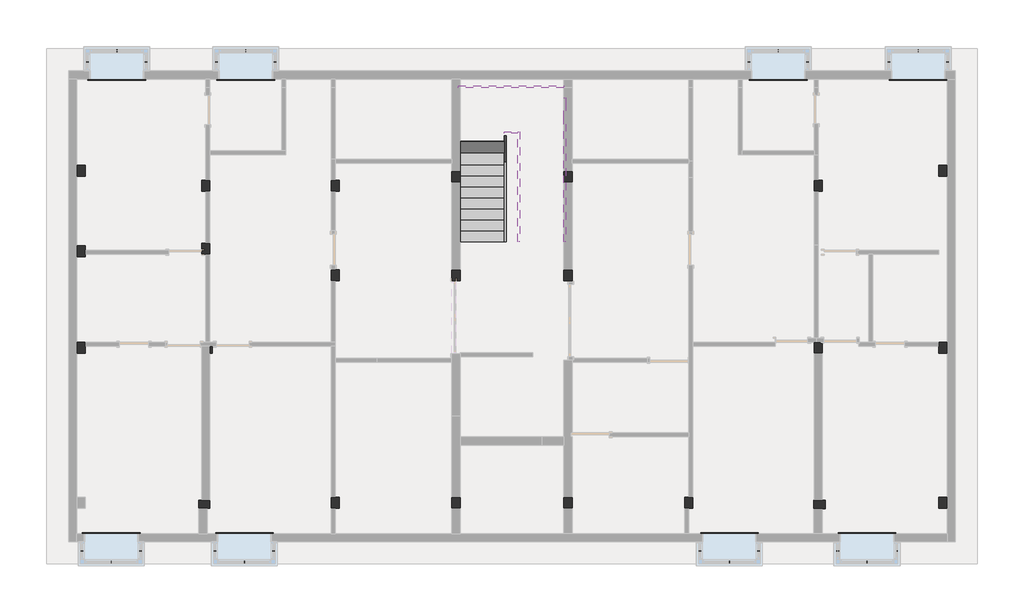
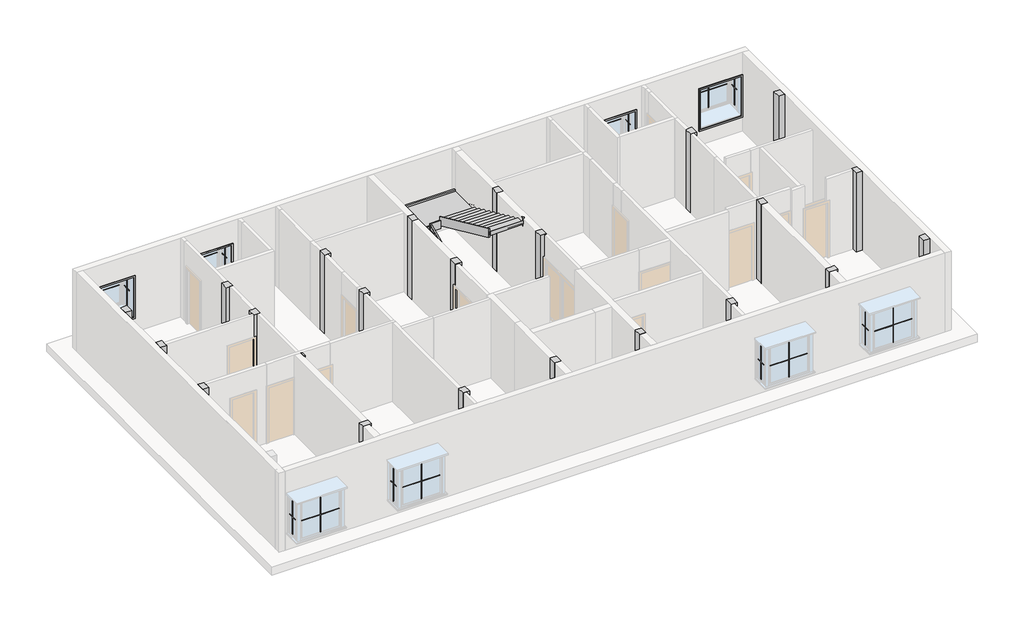
# One storey, part 3 of 3: 32 proxies, 23 columns, 6 members, 1 stair flight.
"""IFC4 building model written with IfcOpenShell, lengths in millimetres."""

from ifc_helpers import new_model, si_unit, frame, origin, place, context, project, spatial, polyline, outline, extrude, faceted_brep, transform, mapped, element, save
from components import m_muntin_pattern_2x2_m_muntin_pattern_2x2_c1fd4460, m_muntin_pattern_2x2_m_muntin_pattern_2x2_777b163a, m_trim_window_interior_flat_picture_frame_44e8afef, stair_flight_7d9339af

model = new_model("IFC4")

# Units and contexts
model_context = context("Model", 3, world=origin())
ifc_project = project(units=[si_unit("LENGTHUNIT", "METRE", prefix="MILLI")], contexts=[model_context])

# Site, building, storey
site = spatial("IfcSite", under=ifc_project)
building = spatial("IfcBuilding", under=site)
storey = spatial("IfcBuildingStorey", under=building, Elevation=19202.4)

# Proxies
placement = place(None, origin())
m_muntin_pattern_2x2_m_muntin_pattern_2x2_shape = m_muntin_pattern_2x2_m_muntin_pattern_2x2_c1fd4460(model_context)
element("IfcBuildingElementProxy", 1, Name="M_Muntin Pattern_2x2 : M_Muntin Pattern_2x2", ObjectType="M_Muntin Pattern_2x2 : M_Muntin Pattern_2x2", at=placement, inside=storey, context=model_context, shape_type="MappedRepresentation", body=[
    mapped(m_muntin_pattern_2x2_m_muntin_pattern_2x2_shape, transform((-11500.7987957, -5499.9182661, 19923.05), x_axis=(-1.0, 0.0, 0.0), y_axis=(0.0, -1.0, 0.0), z_axis=(0.0, 0.0, 1.0))),
])
element("IfcBuildingElementProxy", 2, Name="M_Muntin Pattern_2x2 : M_Muntin Pattern_2x2", ObjectType="M_Muntin Pattern_2x2 : M_Muntin Pattern_2x2", at=placement, inside=storey, context=model_context, shape_type="MappedRepresentation", body=[
    mapped(m_muntin_pattern_2x2_m_muntin_pattern_2x2_shape, transform((-7819.250543, -5499.9182661, 19923.05), x_axis=(-1.0, 0.0, 0.0), y_axis=(0.0, -1.0, 0.0), z_axis=(0.0, 0.0, 1.0))),
])
element("IfcBuildingElementProxy", 3, Name="M_Muntin Pattern_2x2 : M_Muntin Pattern_2x2", ObjectType="M_Muntin Pattern_2x2 : M_Muntin Pattern_2x2", at=placement, inside=storey, context=model_context, shape_type="MappedRepresentation", body=[
    mapped(m_muntin_pattern_2x2_m_muntin_pattern_2x2_shape, transform((5599.7512082, -5499.9182661, 19923.05), x_axis=(-1.0, 0.0, 0.0), y_axis=(0.0, -1.0, 0.0), z_axis=(0.0, 0.0, 1.0))),
])
element("IfcBuildingElementProxy", 4, Name="M_Muntin Pattern_2x2 : M_Muntin Pattern_2x2", ObjectType="M_Muntin Pattern_2x2 : M_Muntin Pattern_2x2", at=placement, inside=storey, context=model_context, shape_type="MappedRepresentation", body=[
    mapped(m_muntin_pattern_2x2_m_muntin_pattern_2x2_shape, transform((9408.6146942, -5499.9182662, 19923.05), x_axis=(-1.0, 0.0, 0.0), y_axis=(0.0, -1.0, 0.0), z_axis=(0.0, 0.0, 1.0))),
])
element("IfcBuildingElementProxy", 5, Name="M_Muntin Pattern_2x2 : M_Muntin Pattern_2x2", ObjectType="M_Muntin Pattern_2x2 : M_Muntin Pattern_2x2", at=placement, inside=storey, context=model_context, shape_type="MappedRepresentation", body=[
    mapped(m_muntin_pattern_2x2_m_muntin_pattern_2x2_shape, transform((-11348.3987957, 8647.7317329, 19923.05), x_axis=(1.0, 0.0, 0.0), y_axis=(0.0, 1.0, 0.0), z_axis=(0.0, 0.0, 1.0))),
])
element("IfcBuildingElementProxy", 6, Name="M_Muntin Pattern_2x2 : M_Muntin Pattern_2x2", ObjectType="M_Muntin Pattern_2x2 : M_Muntin Pattern_2x2", at=placement, inside=storey, context=model_context, shape_type="MappedRepresentation", body=[
    mapped(m_muntin_pattern_2x2_m_muntin_pattern_2x2_shape, transform((-7779.6987993, 8647.7317329, 19923.05), x_axis=(1.0, 0.0, 0.0), y_axis=(0.0, 1.0, 0.0), z_axis=(0.0, 0.0, 1.0))),
])
element("IfcBuildingElementProxy", 7, Name="M_Muntin Pattern_2x2 : M_Muntin Pattern_2x2", ObjectType="M_Muntin Pattern_2x2 : M_Muntin Pattern_2x2", at=placement, inside=storey, context=model_context, shape_type="MappedRepresentation", body=[
    mapped(m_muntin_pattern_2x2_m_muntin_pattern_2x2_shape, transform((6952.301208, 8647.7317329, 19923.05), x_axis=(1.0, 0.0, 0.0), y_axis=(0.0, 1.0, 0.0), z_axis=(0.0, 0.0, 1.0))),
])
element("IfcBuildingElementProxy", 8, Name="M_Muntin Pattern_2x2 : M_Muntin Pattern_2x2", ObjectType="M_Muntin Pattern_2x2 : M_Muntin Pattern_2x2", at=placement, inside=storey, context=model_context, shape_type="MappedRepresentation", body=[
    mapped(m_muntin_pattern_2x2_m_muntin_pattern_2x2_shape, transform((10825.8012075, 8647.7317329, 19923.05), x_axis=(1.0, 0.0, 0.0), y_axis=(0.0, 1.0, 0.0), z_axis=(0.0, 0.0, 1.0))),
])
m_muntin_pattern_2x2_m_muntin_pattern_2x2_2_shape = m_muntin_pattern_2x2_m_muntin_pattern_2x2_777b163a(model_context)
element("IfcBuildingElementProxy", 9, Name="M_Muntin Pattern_2x2 : M_Muntin Pattern_2x2", ObjectType="M_Muntin Pattern_2x2 : M_Muntin Pattern_2x2", at=placement, inside=storey, context=model_context, shape_type="MappedRepresentation", body=[
    mapped(m_muntin_pattern_2x2_m_muntin_pattern_2x2_2_shape, transform((-10690.4737957, -5190.3932661, 19923.05), x_axis=(0.0, 1.0, 0.0), y_axis=(-1.0, 0.0, 0.0), z_axis=(0.0, 0.0, 1.0))),
])
element("IfcBuildingElementProxy", 10, Name="M_Muntin Pattern_2x2 : M_Muntin Pattern_2x2", ObjectType="M_Muntin Pattern_2x2 : M_Muntin Pattern_2x2", at=placement, inside=storey, context=model_context, shape_type="MappedRepresentation", body=[
    mapped(m_muntin_pattern_2x2_m_muntin_pattern_2x2_2_shape, transform((-12311.1237957, -5190.3932661, 19923.05), x_axis=(0.0, -1.0, 0.0), y_axis=(1.0, 0.0, 0.0), z_axis=(0.0, 0.0, 1.0))),
])
element("IfcBuildingElementProxy", 11, Name="M_Muntin Pattern_2x2 : M_Muntin Pattern_2x2", ObjectType="M_Muntin Pattern_2x2 : M_Muntin Pattern_2x2", at=placement, inside=storey, context=model_context, shape_type="MappedRepresentation", body=[
    mapped(m_muntin_pattern_2x2_m_muntin_pattern_2x2_2_shape, transform((-7008.925543, -5190.3932661, 19923.05), x_axis=(0.0, 1.0, 0.0), y_axis=(-1.0, 0.0, 0.0), z_axis=(0.0, 0.0, 1.0))),
])
element("IfcBuildingElementProxy", 12, Name="M_Muntin Pattern_2x2 : M_Muntin Pattern_2x2", ObjectType="M_Muntin Pattern_2x2 : M_Muntin Pattern_2x2", at=placement, inside=storey, context=model_context, shape_type="MappedRepresentation", body=[
    mapped(m_muntin_pattern_2x2_m_muntin_pattern_2x2_2_shape, transform((-8629.575543, -5190.3932661, 19923.05), x_axis=(0.0, -1.0, 0.0), y_axis=(1.0, 0.0, 0.0), z_axis=(0.0, 0.0, 1.0))),
])
element("IfcBuildingElementProxy", 13, Name="M_Muntin Pattern_2x2 : M_Muntin Pattern_2x2", ObjectType="M_Muntin Pattern_2x2 : M_Muntin Pattern_2x2", at=placement, inside=storey, context=model_context, shape_type="MappedRepresentation", body=[
    mapped(m_muntin_pattern_2x2_m_muntin_pattern_2x2_2_shape, transform((6410.0762082, -5190.3932661, 19923.05), x_axis=(0.0, 1.0, 0.0), y_axis=(-1.0, 0.0, 0.0), z_axis=(0.0, 0.0, 1.0))),
])
element("IfcBuildingElementProxy", 14, Name="M_Muntin Pattern_2x2 : M_Muntin Pattern_2x2", ObjectType="M_Muntin Pattern_2x2 : M_Muntin Pattern_2x2", at=placement, inside=storey, context=model_context, shape_type="MappedRepresentation", body=[
    mapped(m_muntin_pattern_2x2_m_muntin_pattern_2x2_2_shape, transform((4789.4262082, -5190.3932661, 19923.05), x_axis=(0.0, -1.0, 0.0), y_axis=(1.0, 0.0, 0.0), z_axis=(0.0, 0.0, 1.0))),
])
element("IfcBuildingElementProxy", 15, Name="M_Muntin Pattern_2x2 : M_Muntin Pattern_2x2", ObjectType="M_Muntin Pattern_2x2 : M_Muntin Pattern_2x2", at=placement, inside=storey, context=model_context, shape_type="MappedRepresentation", body=[
    mapped(m_muntin_pattern_2x2_m_muntin_pattern_2x2_2_shape, transform((10218.9396942, -5190.3932662, 19923.05), x_axis=(0.0, 1.0, 0.0), y_axis=(-1.0, 0.0, 0.0), z_axis=(0.0, 0.0, 1.0))),
])
element("IfcBuildingElementProxy", 16, Name="M_Muntin Pattern_2x2 : M_Muntin Pattern_2x2", ObjectType="M_Muntin Pattern_2x2 : M_Muntin Pattern_2x2", at=placement, inside=storey, context=model_context, shape_type="MappedRepresentation", body=[
    mapped(m_muntin_pattern_2x2_m_muntin_pattern_2x2_2_shape, transform((8598.2896942, -5190.3932661, 19923.05), x_axis=(0.0, -1.0, 0.0), y_axis=(1.0, 0.0, 0.0), z_axis=(0.0, 0.0, 1.0))),
])
element("IfcBuildingElementProxy", 17, Name="M_Muntin Pattern_2x2 : M_Muntin Pattern_2x2", ObjectType="M_Muntin Pattern_2x2 : M_Muntin Pattern_2x2", at=placement, inside=storey, context=model_context, shape_type="MappedRepresentation", body=[
    mapped(m_muntin_pattern_2x2_m_muntin_pattern_2x2_2_shape, transform((-12158.7237957, 8338.2067329, 19923.05), x_axis=(0.0, -1.0, 0.0), y_axis=(1.0, 0.0, 0.0), z_axis=(0.0, 0.0, 1.0))),
])
element("IfcBuildingElementProxy", 18, Name="M_Muntin Pattern_2x2 : M_Muntin Pattern_2x2", ObjectType="M_Muntin Pattern_2x2 : M_Muntin Pattern_2x2", at=placement, inside=storey, context=model_context, shape_type="MappedRepresentation", body=[
    mapped(m_muntin_pattern_2x2_m_muntin_pattern_2x2_2_shape, transform((-10538.0737957, 8338.2067329, 19923.05), x_axis=(0.0, 1.0, 0.0), y_axis=(-1.0, 0.0, 0.0), z_axis=(0.0, 0.0, 1.0))),
])
element("IfcBuildingElementProxy", 19, Name="M_Muntin Pattern_2x2 : M_Muntin Pattern_2x2", ObjectType="M_Muntin Pattern_2x2 : M_Muntin Pattern_2x2", at=placement, inside=storey, context=model_context, shape_type="MappedRepresentation", body=[
    mapped(m_muntin_pattern_2x2_m_muntin_pattern_2x2_2_shape, transform((-8590.0237993, 8338.2067329, 19923.05), x_axis=(0.0, -1.0, 0.0), y_axis=(1.0, 0.0, 0.0), z_axis=(0.0, 0.0, 1.0))),
])
element("IfcBuildingElementProxy", 20, Name="M_Muntin Pattern_2x2 : M_Muntin Pattern_2x2", ObjectType="M_Muntin Pattern_2x2 : M_Muntin Pattern_2x2", at=placement, inside=storey, context=model_context, shape_type="MappedRepresentation", body=[
    mapped(m_muntin_pattern_2x2_m_muntin_pattern_2x2_2_shape, transform((-6969.3737993, 8338.2067329, 19923.05), x_axis=(0.0, 1.0, 0.0), y_axis=(-1.0, 0.0, 0.0), z_axis=(0.0, 0.0, 1.0))),
])
element("IfcBuildingElementProxy", 21, Name="M_Muntin Pattern_2x2 : M_Muntin Pattern_2x2", ObjectType="M_Muntin Pattern_2x2 : M_Muntin Pattern_2x2", at=placement, inside=storey, context=model_context, shape_type="MappedRepresentation", body=[
    mapped(m_muntin_pattern_2x2_m_muntin_pattern_2x2_2_shape, transform((6141.976208, 8338.2067329, 19923.05), x_axis=(0.0, -1.0, 0.0), y_axis=(1.0, 0.0, 0.0), z_axis=(0.0, 0.0, 1.0))),
])
element("IfcBuildingElementProxy", 22, Name="M_Muntin Pattern_2x2 : M_Muntin Pattern_2x2", ObjectType="M_Muntin Pattern_2x2 : M_Muntin Pattern_2x2", at=placement, inside=storey, context=model_context, shape_type="MappedRepresentation", body=[
    mapped(m_muntin_pattern_2x2_m_muntin_pattern_2x2_2_shape, transform((7762.626208, 8338.2067329, 19923.05), x_axis=(0.0, 1.0, 0.0), y_axis=(-1.0, 0.0, 0.0), z_axis=(0.0, 0.0, 1.0))),
])
element("IfcBuildingElementProxy", 23, Name="M_Muntin Pattern_2x2 : M_Muntin Pattern_2x2", ObjectType="M_Muntin Pattern_2x2 : M_Muntin Pattern_2x2", at=placement, inside=storey, context=model_context, shape_type="MappedRepresentation", body=[
    mapped(m_muntin_pattern_2x2_m_muntin_pattern_2x2_2_shape, transform((10015.4762075, 8338.2067329, 19923.05), x_axis=(0.0, -1.0, 0.0), y_axis=(1.0, 0.0, 0.0), z_axis=(0.0, 0.0, 1.0))),
])
element("IfcBuildingElementProxy", 24, Name="M_Muntin Pattern_2x2 : M_Muntin Pattern_2x2", ObjectType="M_Muntin Pattern_2x2 : M_Muntin Pattern_2x2", at=placement, inside=storey, context=model_context, shape_type="MappedRepresentation", body=[
    mapped(m_muntin_pattern_2x2_m_muntin_pattern_2x2_2_shape, transform((11636.1262075, 8338.2067329, 19923.05), x_axis=(0.0, 1.0, 0.0), y_axis=(-1.0, 0.0, 0.0), z_axis=(0.0, 0.0, 1.0))),
])
m_trim_window_interior_flat_picture_frame_shape = m_trim_window_interior_flat_picture_frame_44e8afef(model_context)
element("IfcBuildingElementProxy", 25, Name="M_Trim-Window-Interior-Flat : Picture Frame", ObjectType="M_Trim-Window-Interior-Flat : Picture Frame", at=placement, inside=storey, context=model_context, shape_type="MappedRepresentation", body=[
    mapped(m_trim_window_interior_flat_picture_frame_shape, transform((-11500.7987957, -4712.5932661, 21353.2), x_axis=(-1.0, 0.0, 0.0), y_axis=(0.0, 0.0, 1.0), z_axis=(0.0, 1.0, 0.0))),
])
element("IfcBuildingElementProxy", 26, Name="M_Trim-Window-Interior-Flat : Picture Frame", ObjectType="M_Trim-Window-Interior-Flat : Picture Frame", at=placement, inside=storey, context=model_context, shape_type="MappedRepresentation", body=[
    mapped(m_trim_window_interior_flat_picture_frame_shape, transform((-7819.250543, -4712.5932661, 21353.2), x_axis=(-1.0, 0.0, 0.0), y_axis=(0.0, 0.0, 1.0), z_axis=(0.0, 1.0, 0.0))),
])
element("IfcBuildingElementProxy", 27, Name="M_Trim-Window-Interior-Flat : Picture Frame", ObjectType="M_Trim-Window-Interior-Flat : Picture Frame", at=placement, inside=storey, context=model_context, shape_type="MappedRepresentation", body=[
    mapped(m_trim_window_interior_flat_picture_frame_shape, transform((5599.7512082, -4712.5932661, 21353.2), x_axis=(-1.0, 0.0, 0.0), y_axis=(0.0, 0.0, 1.0), z_axis=(0.0, 1.0, 0.0))),
])
element("IfcBuildingElementProxy", 28, Name="M_Trim-Window-Interior-Flat : Picture Frame", ObjectType="M_Trim-Window-Interior-Flat : Picture Frame", at=placement, inside=storey, context=model_context, shape_type="MappedRepresentation", body=[
    mapped(m_trim_window_interior_flat_picture_frame_shape, transform((9408.6146942, -4712.5932661, 21353.2), x_axis=(-1.0, 0.0, 0.0), y_axis=(0.0, 0.0, 1.0), z_axis=(0.0, 1.0, 0.0))),
])
element("IfcBuildingElementProxy", 29, Name="M_Trim-Window-Interior-Flat : Picture Frame", ObjectType="M_Trim-Window-Interior-Flat : Picture Frame", at=placement, inside=storey, context=model_context, shape_type="MappedRepresentation", body=[
    mapped(m_trim_window_interior_flat_picture_frame_shape, transform((-11348.3987957, 7860.4067329, 21353.2), x_axis=(1.0, 0.0, 0.0), y_axis=(0.0, 0.0, 1.0), z_axis=(0.0, -1.0, 0.0))),
])
element("IfcBuildingElementProxy", 30, Name="M_Trim-Window-Interior-Flat : Picture Frame", ObjectType="M_Trim-Window-Interior-Flat : Picture Frame", at=placement, inside=storey, context=model_context, shape_type="MappedRepresentation", body=[
    mapped(m_trim_window_interior_flat_picture_frame_shape, transform((-7779.6987993, 7860.4067329, 21353.2), x_axis=(1.0, 0.0, 0.0), y_axis=(0.0, 0.0, 1.0), z_axis=(0.0, -1.0, 0.0))),
])
element("IfcBuildingElementProxy", 31, Name="M_Trim-Window-Interior-Flat : Picture Frame", ObjectType="M_Trim-Window-Interior-Flat : Picture Frame", at=placement, inside=storey, context=model_context, shape_type="MappedRepresentation", body=[
    mapped(m_trim_window_interior_flat_picture_frame_shape, transform((6952.301208, 7860.4067329, 21353.2), x_axis=(1.0, 0.0, 0.0), y_axis=(0.0, 0.0, 1.0), z_axis=(0.0, -1.0, 0.0))),
])
element("IfcBuildingElementProxy", 32, Name="M_Trim-Window-Interior-Flat : Picture Frame", ObjectType="M_Trim-Window-Interior-Flat : Picture Frame", at=placement, inside=storey, context=model_context, shape_type="MappedRepresentation", body=[
    mapped(m_trim_window_interior_flat_picture_frame_shape, transform((10825.8012075, 7860.4067329, 21353.2), x_axis=(1.0, 0.0, 0.0), y_axis=(0.0, 0.0, 1.0), z_axis=(0.0, -1.0, 0.0))),
])

# Columns
element("IfcColumn", 33, ObjectType="Rectangular Column : 1'X 9\"", at=placement, inside=storey, context=model_context, shape_type="SweptSolid", body=[
    extrude(outline(polyline([(-12224.6987957, 583.3067334), (-12224.6987957, 278.5067334), (-12453.2987957, 278.5067334), (-12453.2987957, 583.3067334), (-12224.6987957, 583.3067334)])), frame((0.0, 0.0, 19202.4), z_axis=(0.0, 0.0, 1.0), x_axis=(1.0, 0.0, 0.0)), (0.0, 0.0, 1.0), 3048.0),
])
element("IfcColumn", 34, ObjectType="Rectangular Column : 1'X 9\"", at=placement, inside=storey, context=model_context, shape_type="SweptSolid", body=[
    extrude(outline(polyline([(-12224.6987957, 3256.6567332), (-12224.6987957, 2951.8567332), (-12453.2987957, 2951.8567332), (-12453.2987957, 3256.6567332), (-12224.6987957, 3256.6567332)])), frame((0.0, 0.0, 19202.4), z_axis=(0.0, 0.0, 1.0), x_axis=(1.0, 0.0, 0.0)), (0.0, 0.0, 1.0), 3048.0),
])
element("IfcColumn", 35, ObjectType="Rectangular Column : 1'X 9\"", at=placement, inside=storey, context=model_context, shape_type="Brep", body=[
    faceted_brep([(-8770.2987992, 5066.406733, 19202.4), (-8770.2987992, 4761.606733, 19202.4), (-8884.5987992, 4761.606733, 19202.4), (-8998.8987992, 4761.606733, 19202.4), (-8998.8987992, 5066.406733, 19202.4), (-8884.5987992, 5066.406733, 19202.4), (-8770.2987992, 5066.406733, 22250.4), (-8770.2987992, 4761.606733, 22250.4), (-8884.5987992, 4761.606733, 22250.4), (-8998.8987992, 4761.606733, 22250.4), (-8998.8987992, 5066.406733, 22250.4), (-8884.5987992, 5066.406733, 22250.4)], [[[0, 1, 2, 3, 4, 5]], [[6, 7, 1, 0]], [[7, 8, 9, 3, 2, 1]], [[9, 10, 4, 3]], [[10, 11, 6, 0, 5, 4]], [[6, 11, 10, 9, 8, 7]]]),
])
element("IfcColumn", 36, ObjectType="Rectangular Column : 1'X 9\"", at=placement, inside=storey, context=model_context, shape_type="Brep", body=[
    faceted_brep([(-8770.2987992, 3326.5067332, 19202.4), (-8770.2987992, 3021.7067332, 19202.4), (-8884.598796, 3021.7067332, 19202.4), (-8998.8987992, 3021.7067332, 19202.4), (-8998.8987992, 3326.5067332, 19202.4), (-8884.5987992, 3326.5067332, 19202.4), (-8770.2987992, 3326.5067332, 22250.4), (-8770.2987992, 3021.7067332, 22250.4), (-8884.598796, 3021.7067332, 22250.4), (-8998.8987992, 3021.7067332, 22250.4), (-8998.8987992, 3326.5067332, 22250.4), (-8884.5987992, 3326.5067332, 22250.4)], [[[0, 1, 2, 3, 4, 5]], [[6, 7, 1, 0]], [[7, 8, 9, 3, 2, 1]], [[9, 10, 4, 3]], [[10, 11, 6, 0, 5, 4]], [[6, 11, 10, 9, 8, 7]]]),
])
element("IfcColumn", 37, ObjectType="Rectangular Column : 1'X 9\"", at=placement, inside=storey, context=model_context, shape_type="SweptSolid", body=[
    extrude(outline(polyline([(-8713.148796, 278.5067334), (-8771.750543, 278.5067334), (-8771.750543, 469.0067334), (-8713.148796, 469.0067334), (-8713.148796, 278.5067334)])), frame((0.0, 0.0, 19202.4), z_axis=(0.0, 0.0, 1.0), x_axis=(1.0, 0.0, 0.0)), (0.0, 0.0, 1.0), 3048.0),
])
element("IfcColumn", 38, ObjectType="Rectangular Column : 1'X 9\"", at=placement, inside=storey, context=model_context, shape_type="Brep", body=[
    faceted_brep([(-5188.8987995, 5066.406733, 19202.4), (-5188.8987995, 4761.606733, 19202.4), (-5303.1987995, 4761.606733, 19202.4), (-5417.4987995, 4761.606733, 19202.4), (-5417.4987995, 5066.406733, 19202.4), (-5303.1987995, 5066.406733, 19202.4), (-5188.8987995, 5066.406733, 22250.4), (-5188.8987995, 4761.606733, 22250.4), (-5303.1987995, 4761.606733, 22250.4), (-5417.4987995, 4761.606733, 22250.4), (-5417.4987995, 5066.406733, 22250.4), (-5303.1987995, 5066.406733, 22250.4)], [[[0, 1, 2, 3, 4, 5]], [[6, 7, 1, 0]], [[7, 8, 9, 3, 2, 1]], [[9, 10, 4, 3]], [[10, 11, 6, 0, 5, 4]], [[6, 11, 10, 9, 8, 7]]]),
])
element("IfcColumn", 39, ObjectType="Rectangular Column : 1'X 9\"", at=placement, inside=storey, context=model_context, shape_type="Brep", body=[
    faceted_brep([(-5188.8987995, 2589.9067802, 19202.4), (-5188.8987995, 2285.1067802, 19202.4), (-5303.1987995, 2285.1067802, 19202.4), (-5417.4987995, 2285.1067802, 19202.4), (-5417.4987995, 2589.9067802, 19202.4), (-5303.1987995, 2589.9067802, 19202.4), (-5188.8987995, 2589.9067802, 22250.4), (-5188.8987995, 2285.1067802, 22250.4), (-5303.1987995, 2285.1067802, 22250.4), (-5417.4987995, 2285.1067802, 22250.4), (-5417.4987995, 2589.9067802, 22250.4), (-5303.1987995, 2589.9067802, 22250.4)], [[[0, 1, 2, 3, 4, 5]], [[6, 7, 1, 0]], [[7, 8, 9, 3, 2, 1]], [[9, 10, 4, 3]], [[10, 11, 6, 0, 5, 4]], [[6, 11, 10, 9, 8, 7]]]),
])
element("IfcColumn", 40, ObjectType="Rectangular Column : 1'X 9\"", at=placement, inside=storey, context=model_context, shape_type="Brep", body=[
    faceted_brep([(-5188.8987963, -3709.2932193, 19202.4), (-5188.8987963, -4014.0932193, 19202.4), (-5303.1987963, -4014.0932193, 19202.4), (-5417.4987963, -4014.0932193, 19202.4), (-5417.4987963, -3709.2932193, 19202.4), (-5303.1987995, -3709.2932193, 19202.4), (-5188.8987963, -3709.2932193, 22250.4), (-5188.8987963, -4014.0932193, 22250.4), (-5303.1987963, -4014.0932193, 22250.4), (-5417.4987963, -4014.0932193, 22250.4), (-5417.4987963, -3709.2932193, 22250.4), (-5303.1987995, -3709.2932193, 22250.4)], [[[0, 1, 2, 3, 4, 5]], [[6, 7, 1, 0]], [[7, 8, 9, 3, 2, 1]], [[9, 10, 4, 3]], [[10, 11, 6, 0, 5, 4]], [[6, 11, 10, 9, 8, 7]]]),
])
element("IfcColumn", 41, ObjectType="Rectangular Column : 1'X 9\"", at=placement, inside=storey, context=model_context, shape_type="SweptSolid", body=[
    extrude(outline(polyline([(1250.0012085, -3709.2932193), (1250.0012085, -4014.0932193), (1021.4012085, -4014.0932193), (1021.4012085, -3709.2932193), (1250.0012085, -3709.2932193)])), frame((0.0, 0.0, 19202.4), z_axis=(0.0, 0.0, 1.0), x_axis=(1.0, 0.0, 0.0)), (0.0, 0.0, 1.0), 3048.0),
])
element("IfcColumn", 42, ObjectType="Rectangular Column : 1'X 9\"", at=placement, inside=storey, context=model_context, shape_type="Brep", body=[
    faceted_brep([(4590.1012082, -3709.2932193, 19202.4), (4590.1012082, -4014.0932193, 19202.4), (4475.8012082, -4014.0932193, 19202.4), (4361.5012082, -4014.0932193, 19202.4), (4361.5012082, -3709.2932193, 19202.4), (4475.8012082, -3709.2932193, 19202.4), (4590.1012082, -3709.2932193, 22250.4), (4590.1012082, -4014.0932193, 22250.4), (4475.8012082, -4014.0932193, 22250.4), (4361.5012082, -4014.0932193, 22250.4), (4361.5012082, -3709.2932193, 22250.4), (4475.8012082, -3709.2932193, 22250.4)], [[[0, 1, 2, 3, 4, 5]], [[6, 7, 1, 0]], [[7, 8, 9, 3, 2, 1]], [[9, 10, 4, 3]], [[10, 11, 6, 0, 5, 4]], [[6, 11, 10, 9, 8, 7]]]),
])
element("IfcColumn", 43, ObjectType="Rectangular Column : 1'X 9\"", at=placement, inside=storey, context=model_context, shape_type="SweptSolid", body=[
    extrude(outline(polyline([(11625.9012075, -3709.2932671), (11625.9012075, -4014.0932671), (11397.3012075, -4014.0932671), (11397.3012075, -3709.2932671), (11625.9012075, -3709.2932671)])), frame((0.0, 0.0, 19202.4), z_axis=(0.0, 0.0, 1.0), x_axis=(1.0, 0.0, 0.0)), (0.0, 0.0, 1.0), 3048.0),
])
element("IfcColumn", 44, ObjectType="Rectangular Column : 1'X 9\"", at=placement, inside=storey, context=model_context, shape_type="Brep", body=[
    faceted_brep([(11625.9012075, 583.3067295, 19202.4), (11625.9012075, 278.5067295, 19202.4), (11397.3012075, 278.5067295, 19202.4), (11397.3012075, 469.0067295, 19202.4), (11397.3012075, 583.3067295, 19202.4), (11625.9012075, 583.3067295, 22250.4), (11625.9012075, 278.5067295, 22250.4), (11397.3012075, 278.5067295, 22250.4), (11397.3012075, 469.0067295, 22250.4), (11397.3012075, 583.3067295, 22250.4)], [[[0, 1, 2, 3, 4]], [[5, 6, 1, 0]], [[6, 7, 2, 1]], [[7, 8, 9, 4, 3, 2]], [[9, 5, 0, 4]], [[5, 9, 8, 7, 6]]]),
])
element("IfcColumn", 45, ObjectType="Rectangular Column : 1'X 9\"", at=placement, inside=storey, context=model_context, shape_type="SweptSolid", body=[
    extrude(outline(polyline([(11625.9012075, 5479.1567329), (11625.9012075, 5174.3567329), (11397.3012075, 5174.3567329), (11397.3012075, 5479.1567329), (11625.9012075, 5479.1567329)])), frame((0.0, 0.0, 19202.4), z_axis=(0.0, 0.0, 1.0), x_axis=(1.0, 0.0, 0.0)), (0.0, 0.0, 1.0), 3048.0),
])
element("IfcColumn", 46, ObjectType="Rectangular Column : 1'X 9\"", at=placement, inside=storey, context=model_context, shape_type="Brep", body=[
    faceted_brep([(8172.5040565, 5065.4824989, 19202.4), (8172.5040565, 4760.6824989, 19202.4), (8057.2012047, 4760.6824989, 19202.4), (7943.9040565, 4760.6824989, 19202.4), (7943.9040565, 5065.4824989, 19202.4), (8058.2040565, 5065.4824989, 19202.4), (8172.5040565, 5065.4824989, 22250.4), (8172.5040565, 4760.6824989, 22250.4), (8057.2012047, 4760.6824989, 22250.4), (7943.9040565, 4760.6824989, 22250.4), (7943.9040565, 5065.4824989, 22250.4), (8058.2040565, 5065.4824989, 22250.4)], [[[0, 1, 2, 3, 4, 5]], [[6, 7, 1, 0]], [[7, 8, 9, 3, 2, 1]], [[9, 10, 4, 3]], [[10, 11, 6, 0, 5, 4]], [[6, 11, 10, 9, 8, 7]]]),
])
element("IfcColumn", 47, ObjectType="Rectangular Column : 1'X 9\"", at=placement, inside=storey, context=model_context, shape_type="Brep", body=[
    faceted_brep([(8171.5012047, 583.3067334, 19202.4), (8171.5012047, 278.5067334, 19202.4), (7942.9012047, 278.5067334, 19202.4), (7942.9012047, 583.3067334, 19202.4), (8000.0512079, 583.3067334, 19202.4), (8171.5012047, 583.3067334, 22250.4), (8171.5012047, 278.5067334, 22250.4), (7942.9012047, 278.5067334, 22250.4), (7942.9012047, 583.3067334, 22250.4), (8000.0512079, 583.3067334, 22250.4)], [[[0, 1, 2, 3, 4]], [[5, 6, 1, 0]], [[6, 7, 2, 1]], [[7, 8, 3, 2]], [[8, 9, 5, 0, 4, 3]], [[5, 9, 8, 7, 6]]]),
])
element("IfcColumn", 48, ObjectType="Rectangular Column : 1'X 9\"", at=placement, inside=storey, context=model_context, shape_type="Brep", body=[
    faceted_brep([(-9076.550543, -3785.4932196, 19202.4), (-9000.350543, -3785.4932196, 19202.4), (-8771.750543, -3785.4932196, 19202.4), (-8771.750543, -4014.0932196, 19202.4), (-8847.950543, -4014.0932196, 19202.4), (-9076.550543, -4014.0932196, 19202.4), (-9076.550543, -3785.4932196, 22250.4), (-9000.350543, -3785.4932196, 22250.4), (-8771.750543, -3785.4932196, 22250.4), (-8771.750543, -4014.0932196, 22250.4), (-8847.950543, -4014.0932196, 22250.4), (-9076.550543, -4014.0932196, 22250.4)], [[[0, 1, 2, 3, 4, 5]], [[6, 7, 8, 2, 1, 0]], [[8, 9, 3, 2]], [[9, 10, 11, 5, 4, 3]], [[11, 6, 0, 5]], [[6, 11, 10, 9, 8, 7]]]),
])
element("IfcColumn", 49, ObjectType="Rectangular Column : 1'X 9\"", at=placement, inside=storey, context=model_context, shape_type="Brep", body=[
    faceted_brep([(7941.7646942, -3787.3914801, 19202.4), (8246.5646942, -3787.3914801, 19202.4), (8246.5646942, -4015.9914801, 19202.4), (8170.3646942, -4015.9914801, 19202.4), (7941.7646942, -4015.9914801, 19202.4), (7941.7646942, -3787.3914801, 22250.4), (8246.5646942, -3787.3914801, 22250.4), (8246.5646942, -4015.9914801, 22250.4), (8170.3646942, -4015.9914801, 22250.4), (7941.7646942, -4015.9914801, 22250.4)], [[[0, 1, 2, 3, 4]], [[5, 6, 1, 0]], [[6, 7, 2, 1]], [[7, 8, 9, 4, 3, 2]], [[9, 5, 0, 4]], [[5, 9, 8, 7, 6]]]),
])
element("IfcColumn", 50, ObjectType="Rectangular Column : 1'X 9\"", at=placement, inside=storey, context=model_context, shape_type="SweptSolid", body=[
    extrude(outline(polyline([(-12453.2987957, 5174.3567339), (-12453.2987957, 5479.1567339), (-12224.6987957, 5479.1567339), (-12224.6987957, 5174.3567339), (-12453.2987957, 5174.3567339)])), frame((0.0, 0.0, 19202.4), z_axis=(0.0, 0.0, 1.0), x_axis=(1.0, 0.0, 0.0)), (0.0, 0.0, 1.0), 3048.0),
])
element("IfcColumn", 51, ObjectType="Rectangular Column : 1'X 9\"", at=placement, inside=storey, context=model_context, shape_type="SweptSolid", body=[
    extrude(outline(polyline([(-1845.5417538, 5320.4067329), (-1845.5417538, 5015.6067329), (-2074.1417538, 5015.6067329), (-2074.1417538, 5320.4067329), (-1845.5417538, 5320.4067329)])), frame((0.0, 0.0, 19202.4), z_axis=(0.0, 0.0, 1.0), x_axis=(1.0, 0.0, 0.0)), (0.0, 0.0, 1.0), 3048.0),
])
element("IfcColumn", 52, ObjectType="Rectangular Column : 1'X 9\"", at=placement, inside=storey, context=model_context, shape_type="SweptSolid", body=[
    extrude(outline(polyline([(1250.0012085, 5320.4067329), (1250.0012085, 5015.6067329), (1021.4012085, 5015.6067329), (1021.4012085, 5320.4067329), (1250.0012085, 5320.4067329)])), frame((0.0, 0.0, 19202.4), z_axis=(0.0, 0.0, 1.0), x_axis=(1.0, 0.0, 0.0)), (0.0, 0.0, 1.0), 3048.0),
])
element("IfcColumn", 53, ObjectType="Rectangular Column : 1'X 9\"", at=placement, inside=storey, context=model_context, shape_type="SweptSolid", body=[
    extrude(outline(polyline([(-1845.5417538, 2589.906774), (-1845.5417538, 2285.106774), (-2074.1417538, 2285.106774), (-2074.1417538, 2589.906774), (-1845.5417538, 2589.906774)])), frame((0.0, 0.0, 19202.4), z_axis=(0.0, 0.0, 1.0), x_axis=(1.0, 0.0, 0.0)), (0.0, 0.0, 1.0), 3048.0),
])
element("IfcColumn", 54, ObjectType="Rectangular Column : 1'X 9\"", at=placement, inside=storey, context=model_context, shape_type="Brep", body=[
    faceted_brep([(1253.2582462, 2589.9067742, 19202.4), (1253.2582462, 2285.1067742, 19202.4), (1024.6582462, 2285.1067742, 19202.4), (1024.6582462, 2589.9067742, 19202.4), (1250.0012085, 2589.9067742, 19202.4), (1253.2582462, 2589.9067742, 22250.4), (1253.2582462, 2285.1067742, 22250.4), (1024.6582462, 2285.1067742, 22250.4), (1024.6582462, 2589.9067742, 22250.4), (1250.0012085, 2589.9067742, 22250.4)], [[[0, 1, 2, 3, 4]], [[5, 6, 1, 0]], [[6, 7, 2, 1]], [[7, 8, 3, 2]], [[8, 9, 5, 0, 4, 3]], [[5, 9, 8, 7, 6]]]),
])
element("IfcColumn", 55, ObjectType="Rectangular Column : 1'X 9\"", at=placement, inside=storey, context=model_context, shape_type="SweptSolid", body=[
    extrude(outline(polyline([(-1848.7987998, -3709.2932663), (-1848.7987998, -4014.0932663), (-2077.3987998, -4014.0932663), (-2077.3987998, -3709.2932663), (-1848.7987998, -3709.2932663)])), frame((0.0, 0.0, 19202.4), z_axis=(0.0, 0.0, 1.0), x_axis=(1.0, 0.0, 0.0)), (0.0, 0.0, 1.0), 3048.0),
])

# Members
element("IfcMember", 56, ObjectType="Stringer - 2\" Width", at=placement, inside=storey, context=model_context, shape_type="SweptSolid", body=[
    extrude(outline(polyline([(3364.6067329, 19202.4), (3364.6067329, 19402.2262721), (6445.4289342, 20802.6), (7182.0114168, 20802.6), (3661.5714168, 19202.4), (3364.6067329, 19202.4)])), frame((-1896.3417538, 0.0, 0.0), z_axis=(1.0, 0.0, 0.0), x_axis=(0.0, 1.0, 0.0)), (0.0, 0.0, 1.0), 50.8),
])
element("IfcMember", 57, ObjectType="Stringer - 2\" Width", at=placement, inside=storey, context=model_context, shape_type="SweptSolid", body=[
    extrude(outline(polyline([(-1896.3417538, 7631.8067329), (-1896.3417538, 7682.6067329), (1021.4012085, 7682.6067329), (1021.4012085, 7631.8067329), (-1896.3417538, 7631.8067329)])), frame((0.0, 0.0, 20497.8), z_axis=(0.0, 0.0, 1.0), x_axis=(1.0, 0.0, 0.0)), (0.0, 0.0, 1.0), 304.8),
])
element("IfcMember", 58, ObjectType="Stringer - 2\" Width", at=placement, inside=storey, context=model_context, shape_type="SweptSolid", body=[
    extrude(outline(polyline([(6618.562049, 20497.8), (3364.6067329, 21976.8705982), (3364.6067329, 22311.6808176), (7355.1445316, 20497.8), (6618.562049, 20497.8)])), frame((1021.4012085, 0.0, 0.0), z_axis=(1.0, 0.0, 0.0), x_axis=(0.0, 1.0, 0.0)), (0.0, 0.0, 1.0), 50.8),
])
element("IfcMember", 59, ObjectType="Stringer - 2\" Width", at=placement, inside=storey, context=model_context, shape_type="SweptSolid", body=[
    extrude(outline(polyline([(3364.6067329, 19202.4), (3364.6067329, 19402.2262721), (6361.8067329, 20764.5899085), (6361.8067329, 20429.7796892), (3661.5714168, 19202.4), (3364.6067329, 19202.4)])), frame((-629.5987998, 0.0, 0.0), z_axis=(1.0, 0.0, 0.0), x_axis=(0.0, 1.0, 0.0)), (0.0, 0.0, 1.0), 50.8),
])
element("IfcMember", 60, ObjectType="Stringer - 2\" Width", at=placement, inside=storey, context=model_context, shape_type="SweptSolid", body=[
    extrude(outline(polyline([(-629.5987998, 6361.8067329), (-629.5987998, 6412.6067329), (-248.5987915, 6412.6067329), (-248.5987915, 6361.8067329), (-629.5987998, 6361.8067329)])), frame((0.0, 0.0, 20497.8), z_axis=(0.0, 0.0, 1.0), x_axis=(1.0, 0.0, 0.0)), (0.0, 0.0, 1.0), 304.8),
])
element("IfcMember", 61, ObjectType="Stringer - 2\" Width", at=placement, inside=storey, context=model_context, shape_type="SweptSolid", body=[
    extrude(outline(polyline([(6412.6067329, 20926.2262721), (6412.6067329, 20591.4160528), (3364.6067329, 21976.8705982), (3364.6067329, 22311.6808176), (6412.6067329, 20926.2262721)])), frame((-248.5987915, 0.0, 0.0), z_axis=(1.0, 0.0, 0.0), x_axis=(0.0, 1.0, 0.0)), (0.0, 0.0, 1.0), 50.8),
])

# Stair flight
stair_flight_shape = stair_flight_7d9339af(model_context)
element("IfcStairFlight", 62, ObjectType="2\" Tread 1\" Nosing 1/4\" Riser", at=placement, inside=storey, context=model_context, shape_type="MappedRepresentation", body=[
    mapped(stair_flight_shape, transform((0.0, 0.0, 0.0), x_axis=(1.0, 0.0, 0.0), y_axis=(0.0, 1.0, 0.0), z_axis=(0.0, 0.0, 1.0))),
])

save(model, "model.ifc")

# Revit data of these elements
# Type "M_Muntin Pattern_2x2 : M_Muntin Pattern_2x2"
#   Width [instance default] = 3' - 11.24409"
#   Thickness = 0' - 0 1/2"
#   Height [instance default] = 3' - 11.24409"
#   Distance = 0' - 0 3/4"
#   Interior Material [instance default] = none
#   Exterior Material [instance default] = none
#   Default Elevation = 0
# Type "M_Trim-Window-Interior-Flat : Picture Frame"
#   Trim Thickness_Picture Frame = 0' - 1.1811"
#   Trim Width = 0' - 2.3622"
#   Trim Thickness_with Sill = 0' - 0.7874"
#   Sill Thickness = 0' - 1.1811"
#   Opening Width [instance default] = 1' - 11.62205"
#   Opening Height [instance default] = 2' - 11.43307"
#   Default Elevation = 3' - 11.24409"
#   Sill = no
#   Picture Frame = yes
#   Trim Material [instance default] = none
# Type "Rectangular Column : 1'X 9\""
#   Assembly Code = "B1010200"
#   Depth = 1' - 0"
#   Offset Base = 0' - 0"
#   Offset Top = 0' - 0"
#   Width = 0' - 9"
#   Material = none
# Elements 1, 2, 3, 4, 5, 6, 7, 8 (IfcBuildingElementProxy, "M_Muntin Pattern_2x2 : M_Muntin Pattern_2x2")
#   Width = 4' - 5.55512"
#   Height = 4' - 5.55512"
#   Interior Material = Wood - Stained
#   Exterior Material = Clad - White
#   Phase Created = New Construction
#   Materials on its faces: "Clad - White", "Wood - Stained"
# Elements 9, 10, 11, 12, 13, 14, 15, 16, 17, 18, 19, 20, 21, 22, 23, 24 (IfcBuildingElementProxy, "M_Muntin Pattern_2x2 : M_Muntin Pattern_2x2")
#   Width = 1' - 2.12205"
#   Height = 4' - 5.55512"
#   Interior Material = Wood - Stained
#   Exterior Material = Clad - White
#   Phase Created = New Construction
#   Materials on its faces: "Clad - White", "Wood - Stained"
# Elements 25, 26, 27, 28, 29, 30, 31, 32 (IfcBuildingElementProxy, "M_Trim-Window-Interior-Flat : Picture Frame")
#   Opening Width = 4' - 11.05512"
#   Opening Height = 5' - 1.05512"
#   Trim Material = Wood - Stained
#   Phase Created = New Construction
#   Materials on its faces: "Wood - Stained"
# Elements 33, 34, 35, 36, 37, 38, 39, 40, 41, 42, 43, 44, 45, 46, 47, 48, 49, 50, 51, 52, 53, 55 (IfcColumn, "Rectangular Column : 1'X 9\"")
#   Phase Created = New Construction
#   Materials on its faces: "Default Wall"
# Element 54 (IfcColumn, "Rectangular Column : 1'X 9\"")
#   Phase Created = New Construction
# Elements 56, 57, 58, 59, 60, 61 (IfcMember, "Stringer - 2\" Width")
#   Phase Created = New Construction
# Element 62 (IfcStairFlight, "2\" Tread 1\" Nosing 1/4\" Riser")
#   Phase Created = New Construction
# Materials
#   "Clad - White": class "Wood", colour RGB 242 242 238, transparency 0, Cost = 0
#   "Wood - Stained": class "Wood", colour RGB 224 178 126, transparency 0, Cost = 0
#   "Default Wall": colour RGB 128 128 128, transparency 0, Cost = 0
